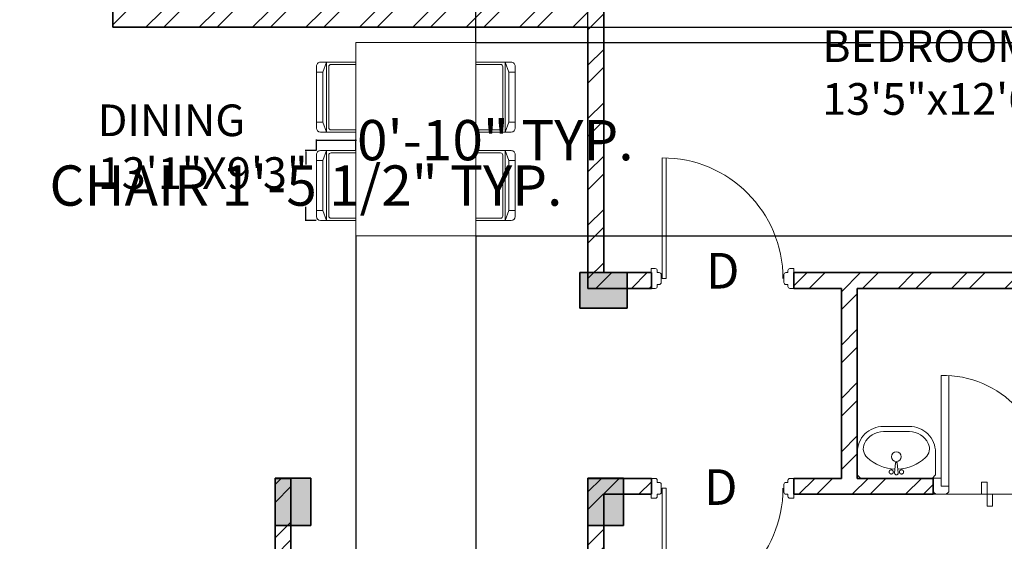
# Model space of a CAD drawing. Units: inches. Extents: x 2379 to 3013, y 1431 to 2110.
# Tile 5 of 10: x 2620 to 2869, y 1795 to 1927. Entities that reach past the tile are written whole.
import ezdxf

# ---------------------------------------------------------------- set-up
doc = ezdxf.new("R2010")
doc.units = ezdxf.units.IN
for name, color, linetype, lineweight in [('00 FURNITURE', 15, 'Continuous', 15), ('A-ANNO-DIMS', 2, 'Continuous', 18), ('A-ANNO-TEXT', 7, 'Continuous', 18), ('A-AREA-IDEN', 7, 'Continuous', 18), ('A-COLS', 7, 'Continuous', 35), ('A-COLS-PATT', 252, 'Continuous', 13), ('A-DOOR', 4, 'Continuous', 18), ('A-FLOR-FIXT', 9, 'Continuous', 18), ('A-WALL-PATT', 8, 'Continuous', 13), ('A_FUR 1', 5, 'Continuous', 5), ('WALL', 7, 'Continuous', 35)]:
    doc.layers.add(name, color=color, linetype=linetype, lineweight=lineweight)
doc.styles.get("Standard").update_dxf_attribs({"font": 'arial.ttf'})
doc.dimstyles.get("Standard").update_dxf_attribs({"dimtxt": 10.18, "dimasz": 0.18, "dimexe": 0.18, "dimexo": 0.0625, "dimgap": 0.09, "dimtad": 0, "dimtih": 1, "dimtoh": 1, "dimdec": 0, "dimzin": 0, "dimdsep": 46, "dimlunit": 3, "dimtxsty": 'Standard', "dimcen": 0.09, "dimadec": 0, "dimazin": 0, "dimtfac": 1, "dimtdec": 0, "dimtofl": 0, "dimtmove": 0, "dimatfit": 3, "dimfxl": 1, "dimtolj": 1, "dimtzin": 0, "dimarcsym": 0})

# ---------------------------------------------------------------- blocks, each defined once
blk = doc.blocks.new('column')
for p, q in [((2588.21, 2021.79), (2597.21, 2021.79)), ((2588.21, 2009.79), (2588.21, 2021.79)), ((2597.21, 2021.79), (2597.21, 2009.79)), ((2597.21, 2009.79), (2588.21, 2009.79))]:
    blk.add_line(p, q)
blk = doc.blocks.new('DDD')
at = {"layer": '00 FURNITURE'}
for p, q in [((-12579.77, -15859.53), (-12579.77, -15829.05)), ((-12578.77, -15859.53), (-12578.77, -15829.03)), ((-12612.02, -15857.03), (-12612.02, -15862.03)), ((-12611.02, -15857.03), (-12612.02, -15857.03)), ((-12610.52, -15858.03), (-12610.52, -15857.53)), ((-12577.52, -15858.03), (-12577.52, -15857.53)), ((-12577.02, -15857.03), (-12576.02, -15857.03)), ((-12576.02, -15857.03), (-12576.02, -15862.03)), ((-12578.77, -15859.53), (-12579.77, -15859.53)), ((-12612.02, -15862.03), (-12611.02, -15862.03)), ((-12610.52, -15861.53), (-12610.52, -15861.03)), ((-12577.52, -15861.53), (-12577.52, -15861.03)), ((-12576.02, -15862.03), (-12577.02, -15862.03))]:
    blk.add_line(p, q, dxfattribs=at)
for points in [[(-12610.52, -15861.03), (-12610.02, -15861.03, 0.414214), (-12609.52, -15860.53), (-12609.52, -15858.53, 0.414214), (-12610.02, -15858.03), (-12610.52, -15858.03)], [(-12577.52, -15861.03), (-12578.02, -15861.03, -0.414214), (-12578.52, -15860.53), (-12578.52, -15858.53, -0.414214), (-12578.02, -15858.03), (-12577.52, -15858.03)]]:
    blk.add_lwpolyline(points, format="xyb", dxfattribs=at)
for centre, radius, start, end in [((-12578.77, -15859.53), 30.5, 90, 180), ((-12611.02, -15857.53), 0.5, 0, 90), ((-12577.02, -15857.53), 0.5, 90, 180), ((-12611.02, -15861.53), 0.5, 270, 0), ((-12577.02, -15861.53), 0.5, 180, 270)]:
    blk.add_arc(centre, radius, start, end, dxfattribs=at)
blk = doc.blocks.new('ESTSET')
at = {"layer": 'A_FUR 1'}
for p, q in [((-10.44, 4.1), (-10.44, 32.1)), ((-8.44, 4.1), (-8.44, 32.1)), ((-36.44, 6.1), (-36.44, 3.1)), ((-34.44, 6.1), (-36.44, 6.1)), ((-34.44, 4.1), (-34.44, 6.1)), ((-34.44, 4.1), (-34.44, 6.1)), ((-8.44, 4.1), (-8.44, 6.1)), ((-8.44, 6.1), (-6.44, 6.1)), ((-8.44, 4.1), (-8.44, 6.1)), ((-6.44, 6.1), (-6.44, 3.1)), ((-32.44, 4.1), (-34.44, 4.1)), ((-32.44, 4.1), (-34.44, 4.1)), ((-32.44, 3.1), (-32.44, 4.1)), ((-10.44, 3.1), (-10.44, 4.1)), ((-10.44, 4.1), (-8.44, 4.1)), ((-10.44, 4.1), (-8.44, 4.1)), ((-6.44, 2.1), (-36.44, 2.1)), ((-35.44, 2.1), (-33.44, 2.1)), ((-7.44, 2.1), (-9.44, 2.1))]:
    blk.add_line(p, q, dxfattribs=at)
for points in [[(-21.44, 2.1), (-18.67, 2.1), (-18.67, 5.1), (-20.06, 5.1)], [(-20.06, 5.1), (-20.06, -0.91)], [(-21.44, 2.1), (-21.44, -0.91), (-20.06, -0.91)]]:
    blk.add_lwpolyline(points, dxfattribs=at)
for centre, radius, start, end in [((-8.91, 6.46), 25.64, 88.9606, 185.2816), ((-35.44, 3.1), 1, 180, 270), ((-33.44, 3.1), 1, 270, 0), ((-9.44, 3.1), 1, 180, 270), ((-7.44, 3.1), 1, 270, 0)]:
    blk.add_arc(centre, radius, start, end, dxfattribs=at)
blk = doc.blocks.new('s_46')
at = {"ltscale": 600}
h = blk.add_hatch(color=256, dxfattribs=at)
edge = h.paths.add_edge_path()
edge.add_line((13.5, 62), (14.2, 54.1))
edge.add_ellipse((4.2, 52.3), major_axis=(-10.1, 0), ratio=1, start_angle=540, end_angle=550.1755, ccw=False)
edge.add_arc((4.2, 52.3), 10.1, 270, 360, ccw=False)
edge.add_line((4.2, 42.2), (4.2, 41.3))
edge.add_line((4.2, 41.3), (11.9, 41.3))
edge.add_arc((4.2, 52.3), 13.4, 664.6981, 766.4848)
h.paths.add_polyline_path([(4.2, 41.3), (-3.4, 41.3, 0.152567), (4.2, 38.9)])
h.paths.add_polyline_path([(11.9, 41.3), (4.2, 41.3), (4.2, 38.9, 0.152567)])
h.paths.add_polyline_path([(-5.7, 54.1), (-5, 62, 0.475833), (-3.4, 41.3), (4.2, 41.3), (4.2, 42.2, -0.46724)])
for p, q in [((-5.9, 52.3), (-0.7, 110.5)), ((-5.9, 52.3), (-0.7, 110.5)), ((9.1, 110.5), (14.2, 54.1)), ((14.3, 52.3), (9.1, 110.5)), ((14.2, 54.1), (14.3, 52.3))]:
    blk.add_line(p, q, dxfattribs=at)
blk.add_lwpolyline([(-220.8, 171.3, -0.414214), (-70.8, 321.3), (79.2, 321.3, -0.414214), (229.2, 171.3), (229.2, 41.3), (209.2, 21.3), (-200.8, 21.3), (-220.8, 41.3)], format="xyb", close=True, dxfattribs=at)
blk.add_lwpolyline([(12.3, 75.4, 0.181638), (172.2, 141.5, 0.326351), (187.7, 222.7, 0.289814), (79.2, 291.3), (-70.8, 291.3, 0.289814), (-179.2, 222.7, 0.326351), (-163.8, 141.5, 0.181638), (-3.8, 75.4)], format="xyb", dxfattribs=at)
for points in [[(-16.8, 67.4), (-17, 67.5), (-17.2, 67.6), (-17.4, 67.6), (-17.6, 67.7), (-17.8, 67.8), (-18, 67.9), (-18.1, 68.1), (-18.2, 68.2), (-18.3, 68.4), (-18.4, 68.6), (-18.5, 68.8), (-18.7, 68.9), (-18.8, 69.1), (-18.9, 69.2), (-19.1, 69.3), (-19.3, 69.3), (-19.5, 69.3), (-19.7, 69.4), (-19.9, 69.4), (-20.1, 69.4), (-20.3, 69.4), (-20.5, 69.5), (-20.7, 69.6), (-20.8, 69.7), (-21, 69.9), (-21.1, 70), (-21.3, 70.2), (-21.4, 70.3), (-21.5, 70.4), (-21.7, 70.5), (-21.9, 70.5), (-22.1, 70.5), (-22.3, 70.5), (-22.5, 70.5), (-22.7, 70.4), (-22.9, 70.4), (-23.1, 70.4), (-23.3, 70.4), (-23.5, 70.5), (-23.7, 70.6), (-23.9, 70.7), (-24, 70.8), (-24.2, 70.9), (-24.4, 71), (-24.6, 71.1), (-24.7, 71.1), (-24.9, 71.1), (-25.1, 71), (-25.3, 71), (-25.5, 70.9), (-25.7, 70.8), (-25.9, 70.7), (-26.1, 70.6), (-26.3, 70.6), (-26.5, 70.6), (-26.7, 70.6), (-26.9, 70.7), (-27.1, 70.8), (-27.3, 70.8), (-27.5, 70.9), (-27.7, 70.9), (-27.8, 70.9), (-28, 70.8), (-28.2, 70.8), (-28.3, 70.6), (-28.5, 70.5), (-28.7, 70.4), (-28.9, 70.3), (-29.1, 70.2), (-29.3, 70.1), (-29.6, 70.1), (-29.9, 70.1), (-30.2, 70.1), (-30.5, 70), (-30.8, 69.8), (-31.1, 69.5), (-31.4, 69), (-31.6, 68.4), (-32.3, 68.5), (-32.8, 68.4), (-33.2, 68.3), (-33.5, 68.1), (-33.7, 67.8), (-33.9, 67.6), (-34, 67.3), (-34.1, 67.1), (-34.3, 66.9), (-34.5, 66.7), (-34.7, 66.6), (-34.9, 66.5), (-35.1, 66.4), (-35.2, 66.3), (-35.4, 66.2), (-35.5, 66), (-35.6, 65.9), (-35.6, 65.7), (-35.7, 65.5), (-35.7, 65.3), (-35.7, 65.1), (-35.8, 64.9), (-35.8, 64.7), (-35.9, 64.5), (-36, 64.3), (-36.2, 64.2), (-36.3, 64), (-36.5, 63.9), (-36.6, 63.8), (-36.8, 63.6), (-36.9, 63.5), (-37, 63.3), (-37, 63.1), (-37, 63), (-37, 62.8), (-37, 62.6), (-37, 62.3), (-37, 62.1), (-37, 61.9), (-37, 61.7), (-37.1, 61.5), (-37.2, 61.4), (-37.3, 61.2), (-37.4, 61), (-37.5, 60.8), (-37.6, 60.7), (-37.7, 60.5), (-37.8, 60.3), (-37.8, 60.1), (-37.7, 60), (-37.7, 59.8), (-37.6, 59.6), (-37.5, 59.4), (-37.4, 59.2), (-37.4, 59), (-37.4, 58.8), (-37.4, 58.6), (-37.4, 58.4), (-37.5, 58.2), (-37.6, 58), (-37.7, 57.8), (-37.7, 57.6), (-37.8, 57.4), (-37.8, 57.2), (-37.7, 57.1), (-37.6, 56.9), (-37.5, 56.7), (-37.4, 56.6), (-37.3, 56.4), (-37.2, 56.2), (-37.1, 56), (-37, 55.8), (-37, 55.6), (-37, 55.4), (-37, 55.2), (-37, 55), (-37, 54.8), (-37, 54.6), (-37, 54.4), (-37, 54.2), (-36.9, 54.1), (-36.8, 53.9), (-36.6, 53.8), (-36.5, 53.7), (-36.3, 53.5), (-36.2, 53.4), (-36, 53.2), (-35.9, 53.1), (-35.8, 52.9), (-35.8, 52.7), (-35.7, 52.5), (-35.7, 52.3), (-35.7, 52.1), (-35.6, 51.9), (-35.6, 51.7), (-35.5, 51.5), (-35.4, 51.4), (-35.2, 51.3), (-35.1, 51.2), (-34.9, 51.1), (-34.7, 51), (-34.5, 50.9), (-34.3, 50.8), (-34.2, 50.7), (-34, 50.5), (-33.9, 50.3), (-33.8, 50.1), (-33.8, 49.9), (-33.7, 49.8), (-33.6, 49.6), (-33.5, 49.4), (-33.4, 49.3), (-33.2, 49.2), (-33.1, 49.1), (-32.9, 49.1), (-32.7, 49), (-32.5, 49), (-32.2, 48.9), (-32.1, 48.9), (-31.9, 48.8), (-31.7, 48.7), (-31.6, 48.5), (-31.4, 48.3), (-31.3, 48.2), (-31.2, 48), (-31.1, 47.9), (-30.9, 47.7), (-30.8, 47.6), (-30.6, 47.6), (-30.4, 47.5), (-30.2, 47.5), (-30, 47.6), (-29.8, 47.6), (-29.6, 47.6), (-29.4, 47.6), (-29.2, 47.5), (-29, 47.4), (-28.8, 47.3), (-28.7, 47.2), (-28.5, 47.1), (-28.3, 46.9), (-28.2, 46.8), (-28, 46.7), (-27.8, 46.7), (-27.7, 46.7), (-27.5, 46.7), (-27.3, 46.7), (-27.1, 46.8), (-26.9, 46.9), (-26.7, 46.9), (-26.5, 47), (-26.3, 47), (-26.1, 46.9), (-25.9, 46.9), (-25.7, 46.8), (-25.5, 46.7), (-25.3, 46.6), (-25.1, 46.5), (-24.9, 46.5), (-24.7, 46.5), (-24.6, 46.5), (-24.4, 46.6), (-24.2, 46.7), (-24, 46.8), (-23.9, 46.9), (-23.7, 47), (-23.5, 47.1), (-23.3, 47.1), (-23.1, 47.2), (-22.9, 47.2), (-22.7, 47.1), (-22.5, 47.1), (-22.3, 47), (-22.1, 47), (-21.9, 47), (-21.7, 47.1), (-21.5, 47.1), (-21.4, 47.2), (-21.3, 47.4), (-21.1, 47.5), (-21, 47.7), (-20.8, 47.8), (-20.7, 48), (-20.5, 48.1), (-20.3, 48.1), (-20.1, 48.2), (-19.9, 48.2), (-19.7, 48.2), (-19.5, 48.2), (-19.3, 48.2), (-19.1, 48.3), (-18.9, 48.4), (-18.8, 48.5), (-18.7, 48.6), (-18.5, 48.8), (-18.4, 49), (-18.3, 49.2), (-18.2, 49.3), (-18.1, 49.5), (-18, 49.7), (-17.8, 49.8), (-17.6, 49.9), (-17.4, 49.9), (-17.2, 50), (-17, 50.1), (-16.8, 50.1), (-16.7, 50.2), (-16.5, 50.3), (-16.4, 50.5), (-16.3, 50.7), (-16.3, 50.8), (-16.2, 51), (-16.2, 51.3), (-16.1, 51.5), (-16, 51.6), (-15.9, 51.8), (-15.8, 52), (-15.6, 52.1), (-15.5, 52.2), (-15.3, 52.3), (-15.1, 52.4), (-15, 52.6), (-14.8, 52.7), (-14.7, 52.8), (-14.7, 53), (-14.6, 53.2), (-14.6, 53.4), (-14.6, 53.6), (-14.6, 53.8), (-14.6, 54), (-14.6, 54.2), (-14.5, 54.4), (-14.4, 54.6), (-14.3, 54.8), (-14.2, 54.9), (-14, 55.1), (-13.9, 55.2), (-13.7, 55.4), (-13.6, 55.5), (-13.6, 55.7), (-13.6, 55.9), (-13.6, 56.1), (-13.6, 56.3), (-13.7, 56.5), (-13.7, 56.7), (-13.8, 56.9), (-13.8, 57.1), (-13.8, 57.3), (-13.7, 57.5), (-13.7, 57.7), (-13.6, 57.9), (-13.5, 58.1), (-13.4, 58.2), (-13.3, 58.4), (-13.2, 58.6), (-13.2, 58.8), (-13.2, 59), (-13.3, 59.1), (-13.4, 59.3), (-13.5, 59.5), (-13.6, 59.7), (-13.7, 59.9), (-13.7, 60.1), (-13.8, 60.3), (-13.8, 60.5), (-13.8, 60.7), (-13.7, 60.9), (-13.7, 61.1), (-13.6, 61.3), (-13.6, 61.5), (-13.6, 61.7), (-13.6, 61.9), (-13.6, 62), (-13.7, 62.2), (-13.9, 62.3), (-14, 62.5), (-14.2, 62.6), (-14.3, 62.8), (-14.4, 63), (-14.5, 63.1), (-14.6, 63.3), (-14.6, 63.5), (-14.6, 63.8), (-14.6, 64), (-14.6, 64.2), (-14.6, 64.4), (-14.7, 64.6), (-14.7, 64.7), (-14.8, 64.9), (-15, 65), (-15.1, 65.1), (-15.3, 65.2), (-15.5, 65.3), (-15.6, 65.5), (-15.8, 65.6), (-15.9, 65.7), (-16, 65.9), (-16.1, 66.1), (-16.2, 66.3), (-16.2, 66.5), (-16.3, 66.7), (-16.3, 66.9), (-16.4, 67.1), (-16.5, 67.2), (-16.7, 67.3)], [(22.1, 61.1), (22, 61.3), (22, 61.5), (22, 61.7), (22, 61.9), (22.1, 62), (22.2, 62.2), (22.3, 62.3), (22.4, 62.5), (22.6, 62.6), (22.7, 62.8), (22.8, 63), (22.9, 63.1), (23, 63.3), (23, 63.5), (23, 63.8), (23, 64), (23, 64.2), (23, 64.4), (23.1, 64.6), (23.1, 64.7), (23.2, 64.9), (23.4, 65), (23.5, 65.1), (23.7, 65.2), (23.9, 65.3), (24.1, 65.5), (24.2, 65.6), (24.4, 65.7), (24.5, 65.9), (24.5, 66.1), (24.6, 66.3), (24.7, 66.5), (24.7, 66.7), (24.8, 66.9), (24.9, 67.1), (25, 67.2), (25.1, 67.3), (25.3, 67.4), (25.4, 67.5), (25.6, 67.6), (25.8, 67.6), (26, 67.7), (26.2, 67.8), (26.4, 67.9), (26.5, 68.1), (26.7, 68.2), (26.8, 68.4), (26.9, 68.6), (27, 68.8), (27.1, 68.9), (27.2, 69.1), (27.3, 69.2), (27.5, 69.3), (27.7, 69.3), (27.9, 69.3), (28.1, 69.4), (28.3, 69.4), (28.5, 69.4), (28.7, 69.4), (28.9, 69.5), (29.1, 69.6), (29.2, 69.7), (29.4, 69.9), (29.5, 70), (29.7, 70.2), (29.8, 70.3), (30, 70.4), (30.1, 70.5), (30.3, 70.5), (30.5, 70.5), (30.7, 70.5), (30.9, 70.5), (31.1, 70.4), (31.3, 70.4), (31.5, 70.4), (31.7, 70.4), (31.9, 70.5), (32.1, 70.6), (32.3, 70.7), (32.5, 70.8), (32.6, 70.9), (32.8, 71), (33, 71.1), (33.2, 71.1), (33.4, 71.1), (33.5, 71), (33.7, 71), (33.9, 70.9), (34.1, 70.8), (34.3, 70.7), (34.5, 70.6), (34.7, 70.6), (34.9, 70.6), (35.1, 70.6), (35.3, 70.7), (35.5, 70.8), (35.7, 70.8), (35.9, 70.9), (36.1, 70.9), (36.3, 70.9), (36.4, 70.8), (36.6, 70.8), (36.8, 70.6), (36.9, 70.5), (37.1, 70.4), (37.3, 70.3), (37.5, 70.2), (37.8, 70.1), (38, 70.1), (38.3, 70.1), (38.6, 70.1), (38.9, 70), (39.2, 69.8), (39.5, 69.5), (39.8, 69), (40.1, 68.4), (40.7, 68.5), (41.3, 68.4), (41.7, 68.3), (42, 68.1), (42.2, 67.8), (42.3, 67.6), (42.4, 67.3), (42.6, 67.1), (42.7, 66.9), (42.9, 66.7), (43.1, 66.6), (43.3, 66.5), (43.5, 66.4), (43.6, 66.3), (43.8, 66.2), (43.9, 66), (44, 65.9), (44.1, 65.7), (44.1, 65.5), (44.1, 65.3), (44.2, 65.1), (44.2, 64.9), (44.2, 64.7), (44.3, 64.5), (44.4, 64.3), (44.6, 64.2), (44.7, 64), (44.9, 63.9), (45.1, 63.8), (45.2, 63.6), (45.3, 63.5), (45.4, 63.3), (45.5, 63.1), (45.5, 63), (45.5, 62.8), (45.4, 62.6), (45.4, 62.3), (45.4, 62.1), (45.4, 61.9), (45.4, 61.7), (45.5, 61.5), (45.6, 61.4), (45.7, 61.2), (45.8, 61), (46, 60.8), (46.1, 60.7), (46.1, 60.5), (46.2, 60.3), (46.2, 60.1), (46.1, 60), (46.1, 59.8), (46, 59.6), (45.9, 59.4), (45.9, 59.2), (45.8, 59), (45.8, 58.8), (45.8, 58.6), (45.9, 58.4), (45.9, 58.2), (46, 58), (46.1, 57.8), (46.1, 57.6), (46.2, 57.4), (46.2, 57.2), (46.1, 57.1), (46.1, 56.9), (46, 56.7), (45.8, 56.6), (45.7, 56.4), (45.6, 56.2), (45.5, 56), (45.4, 55.8), (45.4, 55.6), (45.4, 55.4), (45.4, 55.2), (45.4, 55), (45.5, 54.8), (45.5, 54.6), (45.5, 54.4), (45.4, 54.2), (45.3, 54.1), (45.2, 53.9), (45.1, 53.8), (44.9, 53.7), (44.7, 53.5), (44.6, 53.4), (44.4, 53.2), (44.3, 53.1), (44.2, 52.9), (44.2, 52.7), (44.2, 52.5), (44.1, 52.3), (44.1, 52.1), (44.1, 51.9), (44, 51.7), (43.9, 51.5), (43.8, 51.4), (43.6, 51.3), (43.5, 51.2), (43.3, 51.1), (43.1, 51), (42.9, 50.9), (42.7, 50.8), (42.6, 50.7), (42.5, 50.5), (42.4, 50.3), (42.3, 50.1), (42.2, 49.9), (42.1, 49.8), (42, 49.6), (41.9, 49.4), (41.8, 49.3), (41.7, 49.2), (41.5, 49.1), (41.3, 49.1), (41.1, 49), (40.9, 49), (40.7, 48.9), (40.5, 48.9), (40.3, 48.8), (40.1, 48.7), (40, 48.5), (39.9, 48.3), (39.7, 48.2), (39.6, 48), (39.5, 47.9), (39.4, 47.7), (39.2, 47.6), (39, 47.6), (38.8, 47.5), (38.6, 47.5), (38.4, 47.6), (38.2, 47.6), (38, 47.6), (37.8, 47.6), (37.6, 47.5), (37.4, 47.4), (37.2, 47.3), (37.1, 47.2), (36.9, 47.1), (36.8, 46.9), (36.6, 46.8), (36.4, 46.7), (36.3, 46.7), (36.1, 46.7), (35.9, 46.7), (35.7, 46.7), (35.5, 46.8), (35.3, 46.9), (35.1, 46.9), (34.9, 47), (34.7, 47), (34.5, 46.9), (34.3, 46.9), (34.1, 46.8), (33.9, 46.7), (33.7, 46.6), (33.5, 46.5), (33.4, 46.5), (33.2, 46.5), (33, 46.5), (32.8, 46.6), (32.6, 46.7), (32.5, 46.8), (32.3, 46.9), (32.1, 47), (31.9, 47.1), (31.7, 47.1), (31.5, 47.2), (31.3, 47.2), (31.1, 47.1), (30.9, 47.1), (30.7, 47), (30.5, 47), (30.3, 47), (30.1, 47.1), (30, 47.1), (29.8, 47.2), (29.7, 47.4), (29.5, 47.5), (29.4, 47.7), (29.2, 47.8), (29.1, 48), (28.9, 48.1), (28.7, 48.1), (28.5, 48.2), (28.3, 48.2), (28.1, 48.2), (27.9, 48.2), (27.7, 48.2), (27.5, 48.3), (27.3, 48.4), (27.2, 48.5), (27.1, 48.6), (27, 48.8), (26.9, 49), (26.8, 49.2), (26.7, 49.3), (26.5, 49.5), (26.4, 49.7), (26.2, 49.8), (26, 49.9), (25.8, 49.9), (25.6, 50), (25.4, 50.1), (25.3, 50.1), (25.1, 50.2), (25, 50.3), (24.9, 50.5), (24.8, 50.7), (24.7, 50.8), (24.7, 51), (24.6, 51.3), (24.5, 51.5), (24.5, 51.6), (24.4, 51.8), (24.2, 52), (24.1, 52.1), (23.9, 52.2), (23.7, 52.3), (23.5, 52.4), (23.4, 52.6), (23.2, 52.7), (23.1, 52.8), (23.1, 53), (23, 53.2), (23, 53.4), (23, 53.6), (23, 53.8), (23, 54), (23, 54.2), (22.9, 54.4), (22.8, 54.6), (22.7, 54.8), (22.6, 54.9), (22.4, 55.1), (22.3, 55.2), (22.2, 55.4), (22.1, 55.5), (22, 55.7), (22, 55.9), (22, 56.1), (22, 56.3), (22.1, 56.5), (22.1, 56.7), (22.2, 56.9), (22.2, 57.1), (22.2, 57.3), (22.2, 57.5), (22.1, 57.7), (22, 57.9), (21.9, 58.1), (21.8, 58.2), (21.7, 58.4), (21.6, 58.6), (21.6, 58.8), (21.6, 59), (21.7, 59.1), (21.8, 59.3), (21.9, 59.5), (22, 59.7), (22.1, 59.9), (22.2, 60.1), (22.2, 60.3), (22.2, 60.5), (22.2, 60.7), (22.1, 60.9)]]:
    blk.add_lwpolyline(points, close=True, dxfattribs=at)
blk.add_circle((4.2, 146.3), 28, dxfattribs=at)
for centre, radius, start, end in [((4.2, 108.2), 5.42, 24.6783, 155.3217), ((4.2, 52.3), 10.1, 169.8245, 0)]:
    blk.add_arc(centre, radius, start, end, dxfattribs=at)
for centre, major_axis, ratio, start_param, end_param in [((4.2, 110.5), (-4.93, 0), 0.641024, 3.141593, 6.283185), ((4.2, 52.3), (-10.1, 0), 1, 6.10559, 9.602373)]:
    blk.add_ellipse(centre, major_axis=major_axis, ratio=ratio, start_param=start_param, end_param=end_param, dxfattribs=at)
blk = doc.blocks.new('CHAIR-DINING')
for p, q in [((9.93, 17.66), (1.02, 17.66)), ((1.62, 15.13), (2.57, 17.66)), ((2.57, 17.66), (2.57, 0)), ((0, 16.64), (0, 1.02)), ((1.62, 15.13), (1.62, 2.55)), ((3.13, 16.53), (3.13, 1.12)), ((9.93, 17.09), (3.69, 17.09)), ((1.62, 2.55), (2.57, 0)), ((3.69, 0.56), (9.93, 0.56)), ((1.02, 0), (9.93, 0))]:
    blk.add_line(p, q)
blk.add_lwpolyline([(0, 15.13), (0, 2.55), (1.62, 2.55), (1.62, 15.13)], close=True)
for centre, radius, start, end in [((1.02, 16.64), 1.02, 89.9999, 179.9999), ((3.69, 16.53), 0.56, 89.9999, 179.9999), ((1.02, 1.02), 1.02, 179.9999, 269.9999), ((3.69, 1.12), 0.56, 179.9999, 269.9999)]:
    blk.add_arc(centre, radius, start, end)
blk = doc.blocks.new('*D32')
at = {"layer": 'A-ANNO-DIMS', "color": 0, "lineweight": -2, "transparency": 16777216}
for p, q in [((2694.99, 1893.43), (2692.22, 1893.43)), ((2692.4, 1893.25), (2692.4, 1889.96)), ((2692.4, 1875.96), (2692.4, 1879.25)), ((2694.99, 1875.78), (2692.22, 1875.78))]:
    blk.add_line(p, q, dxfattribs=at)
at = {"layer": 'A-ANNO-DIMS', "color": 0, "transparency": 16777216}
for points in [[(2692.37, 1893.25), (2692.43, 1893.25), (2692.4, 1893.43)], [(2692.37, 1875.96), (2692.43, 1875.96), (2692.4, 1875.78)]]:
    blk.add_solid(points, dxfattribs=at)
at = {"layer": 'Defpoints', "color": 0, "transparency": 16777216}
for p in [(2692.4, 1893.43), (2695.05, 1893.43), (2695.05, 1875.78)]:
    blk.add_point(p, dxfattribs=at)
at = {"layer": 'A-ANNO-DIMS', "color": 0, "transparency": 16777216, "insert": (2692.4, 1884.61), "char_height": 10.18, "attachment_point": 5}
blk.add_mtext('\\A1;CHAIR 1\'-5 1/2" TYP.', dxfattribs=at)
blk = doc.blocks.new('*D33')
at = {"layer": 'A-ANNO-DIMS', "color": 0, "lineweight": -2, "transparency": 16777216}
for p, q in [((2695.05, 1893.5), (2695.05, 1896.26)), ((2695.23, 1896.08), (2704.79, 1896.08)), ((2704.97, 1893.5), (2704.97, 1896.26)), ((2704.97, 1896.08), (2705.15, 1896.08))]:
    blk.add_line(p, q, dxfattribs=at)
at = {"layer": 'A-ANNO-DIMS', "color": 0, "transparency": 16777216}
for points in [[(2695.23, 1896.11), (2695.23, 1896.05), (2695.05, 1896.08)], [(2704.79, 1896.11), (2704.79, 1896.05), (2704.97, 1896.08)]]:
    blk.add_solid(points, dxfattribs=at)
at = {"layer": 'Defpoints', "color": 0, "transparency": 16777216}
for p in [(2704.97, 1896.08), (2695.05, 1893.43), (2704.97, 1893.43)]:
    blk.add_point(p, dxfattribs=at)
at = {"layer": 'A-ANNO-DIMS', "color": 0, "transparency": 16777216, "insert": (2740.22, 1896.08), "char_height": 10.18, "attachment_point": 5}
blk.add_mtext('\\A1;0\'-10" TYP.', dxfattribs=at)
blk = doc.blocks.new('*D42')
at = {"layer": 'A-ANNO-DIMS', "color": 0, "lineweight": -2, "transparency": 16777216}
for p, q in [((2731.29, 1945.67), (2731.11, 1945.67)), ((2731.29, 1942.77), (2731.29, 1945.85)), ((2750.86, 1945.67), (2731.47, 1945.67)), ((2751.04, 1942.77), (2751.04, 1945.85))]:
    blk.add_line(p, q, dxfattribs=at)
at = {"layer": 'A-ANNO-DIMS', "color": 0, "transparency": 16777216}
for points in [[(2731.47, 1945.7), (2731.47, 1945.64), (2731.29, 1945.67)], [(2750.86, 1945.7), (2750.86, 1945.64), (2751.04, 1945.67)]]:
    blk.add_solid(points, dxfattribs=at)
at = {"layer": 'Defpoints', "color": 0, "transparency": 16777216}
for p in [(2731.29, 1945.67), (2731.29, 1942.71), (2751.04, 1942.71)]:
    blk.add_point(p, dxfattribs=at)
at = {"layer": 'A-ANNO-DIMS', "color": 0, "transparency": 16777216, "insert": (2665.05, 1945.67), "char_height": 10.18, "attachment_point": 5}
blk.add_mtext('\\A1;BASIN 1\'-7 1/2" TYP.', dxfattribs=at)
blk = doc.blocks.new('*D43')
at = {"layer": 'A-ANNO-DIMS', "color": 0, "lineweight": -2, "transparency": 16777216}
for p, q in [((2751.1, 1942.71), (2754.18, 1942.71)), ((2754, 1942.53), (2754, 1941.33)), ((2751.1, 1929.54), (2754.18, 1929.54)), ((2754, 1929.72), (2754, 1930.92))]:
    blk.add_line(p, q, dxfattribs=at)
at = {"layer": 'A-ANNO-DIMS', "color": 0, "transparency": 16777216}
for points in [[(2753.97, 1942.53), (2754.03, 1942.53), (2754, 1942.71)], [(2753.97, 1929.72), (2754.03, 1929.72), (2754, 1929.54)]]:
    blk.add_solid(points, dxfattribs=at)
at = {"layer": 'Defpoints', "color": 0, "transparency": 16777216}
for p in [(2751.04, 1942.71), (2754, 1942.71), (2751.04, 1929.54)]:
    blk.add_point(p, dxfattribs=at)
at = {"layer": 'A-ANNO-DIMS', "color": 0, "transparency": 16777216, "insert": (2754, 1936.12), "char_height": 10.18, "attachment_point": 5}
blk.add_mtext('\\A1;1\'-1" TYP.', dxfattribs=at)
blk = doc.blocks.new('*D53')
at = {"layer": 'A-ANNO-DIMS', "color": 0, "lineweight": -2, "transparency": 16777216}
for p, q in [((2704.97, 1871.8), (2704.97, 1446.07)), ((2735.32, 1871.8), (2735.32, 1446.07)), ((2705.15, 1446.25), (2735.14, 1446.25)), ((2735.32, 1446.25), (2735.5, 1446.25))]:
    blk.add_line(p, q, dxfattribs=at)
at = {"layer": 'A-ANNO-DIMS', "color": 0, "transparency": 16777216}
for points in [[(2705.15, 1446.28), (2705.15, 1446.22), (2704.97, 1446.25)], [(2735.14, 1446.28), (2735.14, 1446.22), (2735.32, 1446.25)]]:
    blk.add_solid(points, dxfattribs=at)
at = {"layer": 'Defpoints', "color": 0, "transparency": 16777216}
for p in [(2704.97, 1871.87), (2735.32, 1871.87), (2735.32, 1446.25)]:
    blk.add_point(p, dxfattribs=at)
at = {"layer": 'A-ANNO-DIMS', "color": 0, "transparency": 16777216, "insert": (2761.07, 1446.25), "char_height": 10.18, "attachment_point": 5}
blk.add_mtext('\\A1;2\'-6 1/2"', dxfattribs=at)
blk = doc.blocks.new('*D54')
at = {"layer": 'A-ANNO-DIMS', "color": 0, "lineweight": -2, "transparency": 16777216}
for p, q in [((2735.39, 1920.79), (2980.8, 1920.79)), ((2980.62, 1920.61), (2980.62, 1901.53)), ((2980.62, 1872.05), (2980.62, 1891.13)), ((2735.39, 1871.87), (2980.8, 1871.87))]:
    blk.add_line(p, q, dxfattribs=at)
at = {"layer": 'A-ANNO-DIMS', "color": 0, "transparency": 16777216}
for points in [[(2980.59, 1920.61), (2980.65, 1920.61), (2980.62, 1920.79)], [(2980.59, 1872.05), (2980.65, 1872.05), (2980.62, 1871.87)]]:
    blk.add_solid(points, dxfattribs=at)
at = {"layer": 'Defpoints', "color": 0, "transparency": 16777216}
for p in [(2735.32, 1920.79), (2980.62, 1920.79), (2735.32, 1871.87)]:
    blk.add_point(p, dxfattribs=at)
at = {"layer": 'A-ANNO-DIMS', "color": 0, "transparency": 16777216, "insert": (2980.62, 1896.33), "char_height": 10.18, "attachment_point": 5}
blk.add_mtext('\\A1;4\'-1"', dxfattribs=at)
blk = doc.blocks.new('*D65')
at = {"layer": 'A-ANNO-DIMS', "color": 0, "lineweight": -2, "transparency": 16777216}
for p, q in [((2735.32, 1920.86), (2735.32, 2094.64)), ((2735.5, 2094.46), (2763.45, 2094.46)), ((2763.63, 1924.67), (2763.63, 2094.64)), ((2763.63, 2094.46), (2763.81, 2094.46))]:
    blk.add_line(p, q, dxfattribs=at)
at = {"layer": 'A-ANNO-DIMS', "color": 0, "transparency": 16777216}
for points in [[(2735.5, 2094.49), (2735.5, 2094.43), (2735.32, 2094.46)], [(2763.45, 2094.49), (2763.45, 2094.43), (2763.63, 2094.46)]]:
    blk.add_solid(points, dxfattribs=at)
at = {"layer": 'Defpoints', "color": 0, "transparency": 16777216}
for p in [(2763.63, 2094.46), (2763.63, 1924.61), (2735.32, 1920.79)]:
    blk.add_point(p, dxfattribs=at)
at = {"layer": 'A-ANNO-DIMS', "color": 0, "transparency": 16777216, "insert": (2789.38, 2094.46), "char_height": 10.18, "attachment_point": 5}
blk.add_mtext('\\A1;2\'-4 1/2"', dxfattribs=at)
blk = doc.blocks.new('*D66')
at = {"layer": 'A-ANNO-DIMS', "color": 0, "lineweight": -2, "transparency": 16777216}
for p, q in [((2763.69, 1924.61), (2980.8, 1924.61)), ((2980.62, 1924.61), (2980.62, 1924.79)), ((2980.62, 1924.79), (2980.8, 1924.79)), ((2980.62, 1920.97), (2980.62, 1924.43)), ((2735.39, 1920.79), (2980.8, 1920.79))]:
    blk.add_line(p, q, dxfattribs=at)
at = {"layer": 'A-ANNO-DIMS', "color": 0, "transparency": 16777216}
for points in [[(2980.59, 1924.43), (2980.65, 1924.43), (2980.62, 1924.61)], [(2980.59, 1920.97), (2980.65, 1920.97), (2980.62, 1920.79)]]:
    blk.add_solid(points, dxfattribs=at)
at = {"layer": 'Defpoints', "color": 0, "transparency": 16777216}
for p in [(2763.63, 1924.61), (2980.62, 1924.61), (2735.32, 1920.79)]:
    blk.add_point(p, dxfattribs=at)
at = {"layer": 'A-ANNO-DIMS', "color": 0, "transparency": 16777216, "insert": (2994.42, 1924.79), "char_height": 10.18, "attachment_point": 5}
blk.add_mtext('\\A1;0\'-4"', dxfattribs=at)

msp = doc.modelspace()

# ---------------------------------------------------------------- hatches: boundary and pattern name
at = {"layer": 'A-COLS-PATT'}
h = msp.add_hatch(color=256, dxfattribs=at)
h.dxf.hatch_style = 1
h.paths.add_polyline_path([(2937.63, 1813.62), (2928.63, 1813.62), (2928.63, 1810.61), (2925.63, 1810.61), (2925.63, 1806.61), (2928.63, 1806.61), (2928.63, 1804.62), (2937.63, 1804.62)])
h.paths.add_polyline_path([(2928.63, 1813.62), (2925.63, 1813.62), (2925.63, 1810.61), (2928.63, 1810.61)], flags=17)
h.paths.add_polyline_path([(2693.63, 1810.71), (2684.63, 1810.71), (2684.63, 1810.61), (2688.63, 1810.61), (2688.63, 1798.71), (2693.63, 1798.71)])
h.paths.add_polyline_path([(2688.63, 1810.61), (2684.63, 1810.61), (2684.63, 1798.71), (2688.63, 1798.71)], flags=17)
h.paths.add_polyline_path([(2772.63, 1806.61), (2767.63, 1806.61), (2767.63, 1798.71), (2772.63, 1798.71)], flags=17)
h.paths.add_polyline_path([(2772.63, 1810.61), (2763.63, 1810.61), (2763.63, 1798.71), (2767.63, 1798.71), (2767.63, 1806.61), (2772.63, 1806.61)])
h.paths.add_polyline_path([(2773.54, 1858.61), (2763.63, 1858.61), (2763.63, 1862.61), (2761.54, 1862.61), (2761.54, 1853.61), (2773.54, 1853.61)])
h.paths.add_polyline_path([(2773.54, 1862.61), (2763.63, 1862.61), (2763.63, 1858.61), (2773.54, 1858.61)], flags=17)
h.paths.add_polyline_path([(2598.8, 1854.61), (2594.63, 1854.61), (2594.63, 1845.61), (2598.8, 1845.61)])
h.paths.add_polyline_path([(2594.63, 1854.61), (2590.63, 1854.61), (2590.63, 1845.61), (2594.63, 1845.61)])
h.paths.add_polyline_path([(2590.63, 1854.61), (2586.8, 1854.61), (2586.8, 1845.61), (2590.63, 1845.61)])
at = {"layer": 'A-WALL-PATT'}
h = msp.add_hatch(dxfattribs=at)
h.set_pattern_fill('ANSI32', color=256)
h.paths.add_polyline_path([(2925.63, 1862.61), (2815.63, 1862.61), (2815.63, 1858.61), (2827.63, 1858.61), (2827.63, 1810.61), (2815.63, 1810.61), (2815.63, 1806.61), (2850.78, 1806.61), (2850.78, 1810.61), (2831.63, 1810.61), (2831.63, 1858.61), (2925.63, 1858.61)])
h.paths.add_polyline_path([(2925.63, 1810.61), (2880.78, 1810.61), (2880.78, 1806.61), (2925.63, 1806.61)], flags=17)
h.paths.add_polyline_path([(2633.75, 1660.61), (2594.63, 1660.61), (2481.63, 1660.61), (2481.63, 1651.61), (2588.63, 1651.61), (2588.63, 1570.61), (2624.28, 1570.61), (2624.28, 1574.61), (2592.63, 1574.61), (2592.63, 1651.61), (2633.75, 1651.61)])
h.paths.add_polyline_path([(2594.63, 1809.61), (2481.63, 1809.61), (2481.63, 1805.61), (2594.63, 1805.61)])
h.paths.add_polyline_path([(2594.63, 2012.61), (2597.21, 2012.61), (2597.21, 2021.61), (2588.21, 2021.61), (2588.21, 2012.61), (2590.63, 2012.61), (2590.63, 1845.61), (2594.63, 1845.61)])
h.paths.add_polyline_path([(2767.63, 2012.61), (2770.27, 2012.61), (2770.27, 2021.61), (2761.27, 2021.61), (2761.27, 2012.61), (2763.63, 2012.61), (2763.63, 1928.61), (2691.63, 1928.61), (2643.63, 1928.61), (2643.63, 1924.61), (2691.63, 1924.61), (2763.63, 1924.61), (2763.63, 1858.61), (2779.63, 1858.61), (2779.63, 1862.61), (2767.63, 1862.61)])
h.paths.add_polyline_path([(2613.63, 2012.61), (2613.63, 2021.61), (2597.21, 2021.61), (2597.21, 2012.61)])
h.paths.add_polyline_path([(2508.33, 2012.61), (2508.33, 2021.61), (2478.63, 2021.61), (2478.63, 2012.61)])
h.paths.add_polyline_path([(2556.33, 2021.61), (2556.33, 2012.61), (2588.21, 2012.61), (2588.21, 2021.61)])
h.paths.add_polyline_path([(2659.15, 2012.61), (2659.15, 2021.61), (2643.63, 2021.61), (2643.63, 1958.61), (2661.63, 1958.61), (2661.63, 1962.61), (2647.63, 1962.61), (2647.63, 2012.61)])
h.paths.add_polyline_path([(2714.17, 2012.61), (2714.17, 2021.61), (2683.15, 2021.61), (2683.15, 2012.61), (2691.63, 2012.61), (2691.63, 1958.61), (2695.63, 1958.61), (2695.63, 2012.61)])
h.paths.add_polyline_path([(2738.17, 2021.61), (2738.17, 2012.61), (2761.27, 2012.61), (2761.27, 2021.61)])
h.paths.add_polyline_path([(2820.76, 2012.61), (2820.76, 2021.61), (2770.27, 2021.61), (2770.27, 2012.61)])
h.paths.add_polyline_path([(2868.76, 2021.61), (2868.76, 2012.61), (2928.63, 2012.61), (2928.63, 2021.61)])
h.paths.add_polyline_path([(2928.63, 1962.9), (2937.63, 1962.9), (2937.63, 2009.61), (2928.63, 2009.61)])
h.paths.add_polyline_path([(2937.63, 1914.9), (2928.63, 1914.9), (2928.63, 1863.8), (2937.63, 1863.8)])
h.paths.add_polyline_path([(2928.63, 1846.59), (2937.63, 1846.59), (2937.63, 1854.8), (2928.63, 1854.8)])
h.paths.add_polyline_path([(2937.63, 1822.59), (2928.63, 1822.59), (2928.63, 1813.62), (2937.63, 1813.62)])
h.paths.add_polyline_path([(2928.63, 1778.48), (2937.63, 1778.48), (2937.63, 1813.62), (2928.63, 1813.62), (2928.63, 1810.61), (2925.63, 1810.61), (2925.63, 1806.61), (2928.63, 1806.61)])
h.paths.add_polyline_path([(2816.22, 1651.61), (2816.22, 1660.61), (2767.63, 1660.61), (2767.63, 1806.61), (2779.63, 1806.61), (2779.63, 1810.61), (2763.63, 1810.61), (2763.63, 1660.61), (2688.63, 1660.61), (2688.63, 1810.61), (2684.63, 1810.61), (2684.63, 1660.61), (2669.75, 1660.61), (2669.75, 1651.61), (2763.63, 1651.61), (2763.63, 1574.61), (2672.28, 1574.61), (2672.28, 1570.61), (2767.63, 1570.61), (2767.63, 1651.61)])
h.paths.add_polyline_path([(2864.22, 1660.61), (2864.22, 1651.61), (2937.63, 1651.61), (2937.63, 1730.48), (2928.63, 1730.48), (2928.63, 1660.61)])
h.paths.add_polyline_path([(2469.63, 1975.19), (2478.63, 1975.19), (2478.63, 2009.61), (2469.63, 2009.61)])
h.paths.add_polyline_path([(2478.63, 1927.19), (2469.63, 1927.19), (2469.63, 1811.02), (2478.63, 1811.02)])
h.paths.add_polyline_path([(2469.63, 1758.04), (2478.63, 1758.04), (2478.63, 1802.02), (2469.63, 1802.02)])
h.paths.add_polyline_path([(2478.63, 1710.04), (2469.63, 1710.04), (2469.63, 1660.61), (2478.63, 1660.61)])

# ---------------------------------------------------------------- linework, layer by layer
at = {"layer": '00 FURNITURE'}
for p, q in [((2704.97, 1871.87), (2704.97, 1920.79)), ((2704.97, 1920.79), (2735.32, 1920.79)), ((2735.32, 1871.87), (2735.32, 1920.79)), ((2704.97, 1871.87), (2735.32, 1871.87))]:
    msp.add_line(p, q, dxfattribs=at)
at = {"layer": 'WALL'}
for p, q in [((2767.63, 2012.61), (2767.63, 1862.61)), ((2643.63, 1928.61), (2643.63, 1924.61)), ((2643.63, 1924.61), (2691.63, 1924.61)), ((2691.63, 1924.61), (2763.63, 1924.61)), ((2763.63, 1924.61), (2763.63, 1858.61)), ((2767.63, 1862.61), (2779.63, 1862.61)), ((2779.63, 1862.61), (2779.63, 1858.61)), ((2815.63, 1862.61), (2815.63, 1858.61)), ((2815.63, 1862.61), (2928.63, 1862.61)), ((2763.63, 1858.61), (2779.63, 1858.61)), ((2815.63, 1858.61), (2827.63, 1858.61)), ((2827.63, 1858.61), (2827.63, 1810.61)), ((2831.63, 1858.61), (2831.63, 1810.61)), ((2831.63, 1858.61), (2928.63, 1858.61)), ((2684.63, 1810.61), (2688.63, 1810.61)), ((2684.63, 1810.61), (2684.63, 1660.61)), ((2688.63, 1810.61), (2688.63, 1660.61)), ((2763.63, 1810.61), (2763.63, 1660.61)), ((2763.63, 1810.61), (2779.63, 1810.61)), ((2779.63, 1810.61), (2779.63, 1806.61)), ((2815.63, 1810.61), (2815.63, 1806.61)), ((2815.63, 1810.61), (2827.63, 1810.61)), ((2831.63, 1810.61), (2850.78, 1810.61)), ((2850.78, 1810.61), (2850.78, 1806.61)), ((2767.63, 1806.61), (2779.63, 1806.61)), ((2767.63, 1806.61), (2767.63, 1660.61)), ((2815.63, 1806.61), (2850.78, 1806.61))]:
    msp.add_line(p, q, dxfattribs=at)

# ---------------------------------------------------------------- block references
at = {"layer": '00 FURNITURE'}
for p in [(2695.05, 1898.11), (2695.05, 1875.78)]:
    msp.add_blockref('CHAIR-DINING', p, dxfattribs=at)
at = {"layer": '00 FURNITURE', "extrusion": (0, 0, -1), "zscale": -1}
for p in [(-2745.25, 1898.11), (-2745.25, 1875.78)]:
    msp.add_blockref('CHAIR-DINING', p, dxfattribs=at)
at = {"layer": 'A-COLS'}
for p, rotation in [((751.75, 4450.82), 270), ((5281.84, 3820.5), 180), ((5360.84, 3820.5), 180)]:
    msp.add_blockref('column', p, dxfattribs=dict(at, rotation=rotation))
at = {"layer": 'A-DOOR', "xscale": -1}
for name, p in [('DDD', (-9796.4, 17720.64)), ('ESTSET', (2844.35, 1804.54))]:
    msp.add_blockref(name, p, dxfattribs=at)
at = {"layer": 'A-DOOR', "rotation": 180}
msp.add_blockref('DDD', (-9796.4, -14051.42), dxfattribs=at)
at = {"layer": 'A-FLOR-FIXT', "xscale": -0.0438792252617072, "yscale": 0.0438792252617072, "zscale": 0.0438792252617072}
msp.add_blockref('s_46', (2841.69, 1809.67), dxfattribs=at)

# ---------------------------------------------------------------- texts
at = {"layer": 'A-ANNO-TEXT', "char_height": 9, "attachment_point": 1}
for insert in [(2793.44, 1867.58), (2792.94, 1812.92)]:
    msp.add_mtext_dynamic_manual_height_columns('D', width=106.8919, gutter_width=12.5, heights=[0], dxfattribs=dict(at, insert=insert))
at = {"layer": 'A-AREA-IDEN', "char_height": 8, "attachment_point": 1}
for s, insert in [('BEDROOM                             13\'5"x12\'6"  ', (2822.77, 1923.82)), ('DINING \\P13\'1"X9\'3"             ', (2639.83, 1905.09))]:
    msp.add_mtext_dynamic_manual_height_columns(s, width=46.1506, gutter_width=12.5, heights=[0], dxfattribs=dict(at, insert=insert))

# ---------------------------------------------------------------- dimensions: what is measured, and where the dimension line sits
at = {"layer": 'A-ANNO-DIMS'}
for base, p1, p2, picture, middle in [((2763.63, 2094.46), (2735.32, 1920.79), (2763.63, 1924.61), '*D65', (2789.38, 2094.46)), ((2735.3226, 1446.2521), (2704.974, 1871.8654), (2735.3226, 1871.8654), '*D53', (2761.0704, 1446.2521))]:
    dim = msp.add_linear_dim(base=base, p1=p1, p2=p2, dimstyle='Standard', override={"dimdec": 1, "dimlfac": 1, "dimrnd": 0, "dimzin": 1, "dimdsep": 46, "dimlunit": 4, "dimfrac": 2}, dxfattribs=at)
    dim.commit()
    dim.dimension.update_dxf_attribs({"geometry": picture, "text_midpoint": middle})
for base, p1, p2, angle, text, picture, middle in [((2731.2925, 1945.6679), (2751.0381, 1942.706), (2731.2925, 1942.706), 180, 'BASIN <> TYP.', '*D42', (2665.0469, 1945.6679)), ((2754, 1942.71), (2751.04, 1929.54), (2751.04, 1942.71), 90, '<> TYP.', '*D43', (2754, 1936.12)), ((2692.3996, 1893.433), (2695.0479, 1875.7778), (2695.0479, 1893.433), 90, 'CHAIR <> TYP.', '*D32', (2692.3996, 1884.6054))]:
    dim = msp.add_linear_dim(base=base, p1=p1, p2=p2, angle=angle, text=text, dimstyle='Standard', override={"dimdec": 1, "dimlfac": 1, "dimrnd": 0, "dimzin": 1, "dimdsep": 46, "dimlunit": 4, "dimfrac": 2}, dxfattribs=at)
    dim.commit()
    dim.dimension.update_dxf_attribs({"geometry": picture, "text_midpoint": middle})
for base, p1, p2, picture, middle in [((2980.62, 1924.61), (2735.32, 1920.79), (2763.63, 1924.61), '*D66', (2994.42, 1924.79)), ((2980.62, 1920.79), (2735.32, 1871.87), (2735.32, 1920.79), '*D54', (2980.62, 1896.33))]:
    dim = msp.add_linear_dim(base=base, p1=p1, p2=p2, angle=90, dimstyle='Standard', override={"dimdec": 1, "dimlfac": 1, "dimrnd": 0, "dimzin": 1, "dimdsep": 46, "dimlunit": 4, "dimfrac": 2}, dxfattribs=at)
    dim.commit()
    dim.dimension.update_dxf_attribs({"geometry": picture, "text_midpoint": middle})
dim = msp.add_linear_dim(base=(2704.97, 1896.08), p1=(2695.05, 1893.43), p2=(2704.97, 1893.43), text='<> TYP.', dimstyle='Standard', override={"dimdec": 1, "dimlfac": 1, "dimrnd": 0, "dimzin": 1, "dimdsep": 46, "dimlunit": 4, "dimfrac": 2}, dxfattribs=at)
dim.commit()
dim.dimension.update_dxf_attribs({"geometry": '*D33', "text_midpoint": (2740.22, 1896.08)})

doc.saveas('drawing.dxf')
